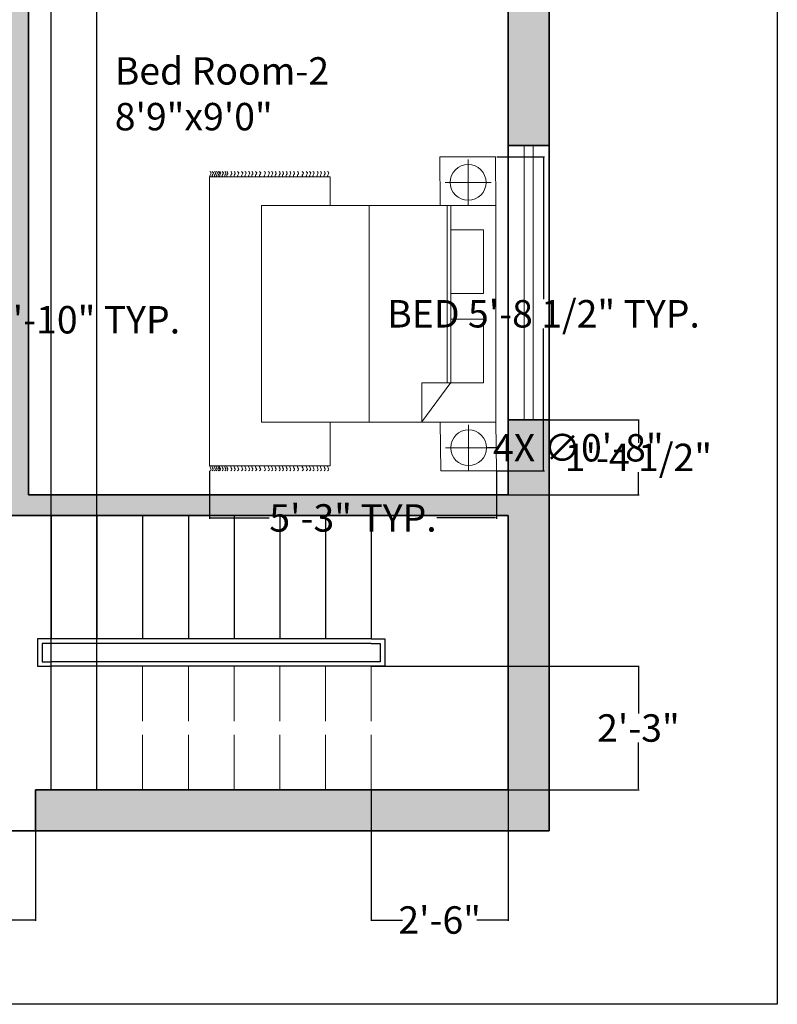
# Model space of a CAD drawing. Units: inches. Extents: x 335 to 688, y 1043 to 1486.
# Tile 2 of 7: x 515 to 681, y 1043 to 1258. Entities that reach past the tile are written whole.
import ezdxf

# ---------------------------------------------------------------- set-up
doc = ezdxf.new("R2010")
doc.units = ezdxf.units.IN
doc.header["$MEASUREMENT"] = 0
doc.linetypes.add('ACAD_ISO02W100', pattern=[15, 12, -3])
for name, color, linetype, lineweight in [('A-ANNO-DIMS', 2, 'Continuous', 18), ('A-ANNO-TTLB', 7, 'Continuous', 25), ('A-AREA-IDEN', 7, 'Continuous', 18), ('A-FLOR-STRS', 7, 'Continuous', 25), ('A-FLOR-STRS-HIDN', 7, 'ACAD_ISO02W100', 18), ('A-FURN', 8, 'Continuous', 18), ('A-GLAZ', 4, 'Continuous', 18), ('A-WALL', 7, 'Continuous', 35), ('A-WALL-PATT', 252, 'Continuous', 13)]:
    doc.layers.add(name, color=color, linetype=linetype, lineweight=lineweight)
doc.styles.get("Standard").update_dxf_attribs({"font": 'arial.ttf'})
doc.dimstyles.get("Standard").update_dxf_attribs({"dimtxt": 6, "dimasz": 0.18, "dimexe": 0.18, "dimexo": 0.0625, "dimgap": 0.09, "dimtad": 0, "dimtih": 1, "dimtoh": 1, "dimdec": 1, "dimzin": 0, "dimdsep": 46, "dimlunit": 3, "dimtxsty": 'Standard', "dimcen": 0.09, "dimadec": 0, "dimazin": 0, "dimtfac": 1, "dimtdec": 1, "dimtofl": 0, "dimtmove": 0, "dimatfit": 3, "dimfxl": 1, "dimtolj": 1, "dimtzin": 0, "dimarcsym": 0})

# ---------------------------------------------------------------- blocks, each defined once
blk = doc.blocks.new('BED-DOUBLE-WITH-NIGHTSTANDS')
for p, q in [((56.59, 58.08), (56.59, 68.14)), ((0, 64.35), (26.37, 64.35)), ((0, 1.12), (0, 64.35)), ((26.37, 64.35), (26.37, 58.06)), ((61.62, 63.11), (51.56, 63.11)), ((34.96, 10.66), (34.96, 58.08)), ((52, 19.27), (52, 58.08)), ((52.82, 19.32), (52.82, 58.08)), ((52.82, 19.32), (46.47, 10.71)), ((52.82, 19.27), (46.47, 19.27)), ((46.47, 19.27), (46.47, 10.71)), ((26.37, 10.66), (26.37, 1.12)), ((56.69, 0.03), (56.69, 10.09)), ((61.72, 5.06), (51.66, 5.06)), ((26.37, 1.12), (0, 1.12))]:
    blk.add_line(p, q)
for points in [[(50.39, 68.71), (50.5, 58.08), (62.68, 58.08), (62.58, 68.71)], [(62.68, 10.66), (11.37, 10.66), (11.37, 58.08), (62.68, 58.08)], [(59.98, 38.83), (52.82, 38.83), (52.82, 52.73), (59.98, 52.73)], [(59.98, 19.27), (52.82, 19.27), (52.82, 33.16), (59.98, 33.16)], [(50.5, 10.66), (50.6, 0.03), (62.78, 0.03), (62.68, 10.66)]]:
    blk.add_lwpolyline(points, close=True)
for centre in [(56.59, 63.11), (56.69, 5.06)]:
    blk.add_circle(centre, 3.92)
for points, knots in [([(0.07, 65.48), (0.19, 65.39), (0.43, 65.19), (0.19, 64.85), (0.02, 64.57), (0.13, 64.42), (0.18, 64.35)], [0, 0, 0, 0, 0.400747, 0.791423, 1.067667, 1.29709, 1.29709, 1.29709, 1.29709]), ([(0.57, 65.48), (0.7, 65.39), (0.94, 65.19), (0.7, 64.85), (0.52, 64.57), (0.63, 64.42), (0.68, 64.35)], [0, 0, 0, 0, 0.400747, 0.791423, 1.067667, 1.29709, 1.29709, 1.29709, 1.29709]), ([(1.06, 65.48), (1.18, 65.39), (1.42, 65.19), (1.18, 64.85), (1.01, 64.57), (1.11, 64.42), (1.16, 64.35)], [0, 0, 0, 0, 0.400747, 0.791423, 1.067667, 1.29709, 1.29709, 1.29709, 1.29709]), ([(1.46, 65.48), (1.58, 65.39), (1.82, 65.19), (1.58, 64.85), (1.41, 64.57), (1.51, 64.42), (1.56, 64.35)], [0, 0, 0, 0, 0.400747, 0.791423, 1.067667, 1.29709, 1.29709, 1.29709, 1.29709]), ([(1.88, 65.48), (2, 65.39), (2.24, 65.19), (2, 64.85), (1.82, 64.57), (1.93, 64.42), (1.98, 64.35)], [0, 0, 0, 0, 0.400747, 0.791423, 1.067667, 1.29709, 1.29709, 1.29709, 1.29709]), ([(2.18, 65.48), (2.31, 65.39), (2.55, 65.19), (2.31, 64.85), (2.13, 64.57), (2.24, 64.42), (2.29, 64.35)], [0, 0, 0, 0, 0.400747, 0.791423, 1.067667, 1.29709, 1.29709, 1.29709, 1.29709]), ([(2.76, 65.48), (2.88, 65.39), (3.12, 65.19), (2.88, 64.85), (2.71, 64.57), (2.81, 64.42), (2.86, 64.35)], [0, 0, 0, 0, 0.400747, 0.791423, 1.067667, 1.29709, 1.29709, 1.29709, 1.29709]), ([(3.33, 65.48), (3.45, 65.39), (3.7, 65.19), (3.44, 64.85), (3.27, 64.57), (3.38, 64.42), (3.43, 64.35)], [0, 0, 0, 0, 0.407265, 0.802015, 1.07826, 1.307683, 1.307683, 1.307683, 1.307683]), ([(3.75, 65.48), (3.88, 65.39), (4.12, 65.19), (3.88, 64.85), (3.7, 64.57), (3.81, 64.42), (3.86, 64.35)], [0, 0, 0, 0, 0.400747, 0.791423, 1.067667, 1.29709, 1.29709, 1.29709, 1.29709]), ([(4.64, 65.48), (4.76, 65.39), (5, 65.19), (4.76, 64.85), (4.59, 64.57), (4.69, 64.42), (4.74, 64.35)], [0, 0, 0, 0, 0.400747, 0.791423, 1.067667, 1.29709, 1.29709, 1.29709, 1.29709]), ([(5.36, 65.48), (5.49, 65.39), (5.73, 65.19), (5.49, 64.85), (5.31, 64.57), (5.42, 64.42), (5.47, 64.35)], [0, 0, 0, 0, 0.400747, 0.791423, 1.067667, 1.29709, 1.29709, 1.29709, 1.29709]), ([(6.12, 65.48), (6.24, 65.39), (6.48, 65.19), (6.24, 64.85), (6.07, 64.57), (6.17, 64.42), (6.22, 64.35)], [0, 0, 0, 0, 0.400747, 0.791423, 1.067667, 1.29709, 1.29709, 1.29709, 1.29709]), ([(7, 65.48), (7.12, 65.39), (7.36, 65.19), (7.12, 64.85), (6.95, 64.57), (7.05, 64.42), (7.1, 64.35)], [0, 0, 0, 0, 0.400747, 0.791423, 1.067667, 1.29709, 1.29709, 1.29709, 1.29709]), ([(7.73, 65.48), (7.85, 65.39), (8.09, 65.19), (7.85, 64.85), (7.68, 64.57), (7.78, 64.42), (7.83, 64.35)], [0, 0, 0, 0, 0.400747, 0.791423, 1.067667, 1.29709, 1.29709, 1.29709, 1.29709]), ([(8.54, 65.48), (8.66, 65.39), (8.9, 65.19), (8.66, 64.85), (8.49, 64.57), (8.6, 64.42), (8.65, 64.35)], [0, 0, 0, 0, 0.400747, 0.791423, 1.067667, 1.29709, 1.29709, 1.29709, 1.29709]), ([(9.23, 65.48), (9.35, 65.39), (9.59, 65.19), (9.35, 64.85), (9.18, 64.57), (9.29, 64.42), (9.34, 64.35)], [0, 0, 0, 0, 0.400747, 0.791423, 1.067667, 1.29709, 1.29709, 1.29709, 1.29709]), ([(10.05, 65.48), (10.17, 65.39), (10.41, 65.19), (10.17, 64.85), (10, 64.57), (10.1, 64.42), (10.15, 64.35)], [0, 0, 0, 0, 0.400747, 0.791423, 1.067667, 1.29709, 1.29709, 1.29709, 1.29709]), ([(10.93, 65.48), (11.05, 65.39), (11.29, 65.19), (11.05, 64.85), (10.88, 64.57), (10.99, 64.42), (11.03, 64.35)], [0, 0, 0, 0, 0.400747, 0.791423, 1.067667, 1.29709, 1.29709, 1.29709, 1.29709]), ([(11.97, 65.48), (12.09, 65.39), (12.33, 65.19), (12.09, 64.85), (11.92, 64.57), (12.02, 64.42), (12.07, 64.35)], [0, 0, 0, 0, 0.400747, 0.791423, 1.067667, 1.29709, 1.29709, 1.29709, 1.29709]), ([(12.85, 65.48), (12.97, 65.39), (13.21, 65.19), (12.97, 64.85), (12.8, 64.57), (12.9, 64.42), (12.95, 64.35)], [0, 0, 0, 0, 0.400747, 0.791423, 1.067667, 1.29709, 1.29709, 1.29709, 1.29709]), ([(13.58, 65.48), (13.7, 65.39), (13.94, 65.19), (13.7, 64.85), (13.53, 64.57), (13.63, 64.42), (13.68, 64.35)], [0, 0, 0, 0, 0.400747, 0.791423, 1.067667, 1.29709, 1.29709, 1.29709, 1.29709]), ([(14.33, 65.48), (14.45, 65.39), (14.69, 65.19), (14.45, 64.85), (14.28, 64.57), (14.38, 64.42), (14.43, 64.35)], [0, 0, 0, 0, 0.400747, 0.791423, 1.067667, 1.29709, 1.29709, 1.29709, 1.29709]), ([(15.21, 65.48), (15.33, 65.39), (15.57, 65.19), (15.33, 64.85), (15.16, 64.57), (15.27, 64.42), (15.32, 64.35)], [0, 0, 0, 0, 0.400747, 0.791423, 1.067667, 1.29709, 1.29709, 1.29709, 1.29709]), ([(15.94, 65.48), (16.06, 65.39), (16.3, 65.19), (16.06, 64.85), (15.89, 64.57), (16, 64.42), (16.04, 64.35)], [0, 0, 0, 0, 0.400747, 0.791423, 1.067667, 1.29709, 1.29709, 1.29709, 1.29709]), ([(16.76, 65.48), (16.88, 65.39), (17.12, 65.19), (16.88, 64.85), (16.7, 64.57), (16.81, 64.42), (16.86, 64.35)], [0, 0, 0, 0, 0.400747, 0.791423, 1.067667, 1.29709, 1.29709, 1.29709, 1.29709]), ([(17.53, 65.48), (17.65, 65.39), (17.89, 65.19), (17.65, 64.85), (17.48, 64.57), (17.59, 64.42), (17.64, 64.35)], [0, 0, 0, 0, 0.400747, 0.791423, 1.067667, 1.29709, 1.29709, 1.29709, 1.29709]), ([(18.35, 65.48), (18.47, 65.39), (18.71, 65.19), (18.47, 64.85), (18.3, 64.57), (18.4, 64.42), (18.45, 64.35)], [0, 0, 0, 0, 0.400747, 0.791423, 1.067667, 1.29709, 1.29709, 1.29709, 1.29709]), ([(19.23, 65.48), (19.35, 65.39), (19.59, 65.19), (19.35, 64.85), (19.18, 64.57), (19.29, 64.42), (19.33, 64.35)], [0, 0, 0, 0, 0.400747, 0.791423, 1.067667, 1.29709, 1.29709, 1.29709, 1.29709]), ([(20.27, 65.48), (20.39, 65.39), (20.63, 65.19), (20.39, 64.85), (20.22, 64.57), (20.32, 64.42), (20.37, 64.35)], [0, 0, 0, 0, 0.400747, 0.791423, 1.067667, 1.29709, 1.29709, 1.29709, 1.29709]), ([(21.15, 65.48), (21.27, 65.39), (21.51, 65.19), (21.27, 64.85), (21.1, 64.57), (21.21, 64.42), (21.25, 64.35)], [0, 0, 0, 0, 0.400747, 0.791423, 1.067667, 1.29709, 1.29709, 1.29709, 1.29709]), ([(21.88, 65.48), (22, 65.39), (22.24, 65.19), (22, 64.85), (21.83, 64.57), (21.93, 64.42), (21.98, 64.35)], [0, 0, 0, 0, 0.400747, 0.791423, 1.067667, 1.29709, 1.29709, 1.29709, 1.29709]), ([(22.63, 65.48), (22.75, 65.39), (22.99, 65.19), (22.75, 64.85), (22.58, 64.57), (22.69, 64.42), (22.73, 64.35)], [0, 0, 0, 0, 0.400747, 0.791423, 1.067667, 1.29709, 1.29709, 1.29709, 1.29709]), ([(23.51, 65.48), (23.63, 65.39), (23.87, 65.19), (23.63, 64.85), (23.46, 64.57), (23.57, 64.42), (23.62, 64.35)], [0, 0, 0, 0, 0.400747, 0.791423, 1.067667, 1.29709, 1.29709, 1.29709, 1.29709]), ([(24.24, 65.48), (24.36, 65.39), (24.6, 65.19), (24.36, 64.85), (24.19, 64.57), (24.3, 64.42), (24.34, 64.35)], [0, 0, 0, 0, 0.400747, 0.791423, 1.067667, 1.29709, 1.29709, 1.29709, 1.29709]), ([(25.06, 65.48), (25.18, 65.39), (25.42, 65.19), (25.18, 64.85), (25.01, 64.57), (25.11, 64.42), (25.16, 64.35)], [0, 0, 0, 0, 0.400747, 0.791423, 1.067667, 1.29709, 1.29709, 1.29709, 1.29709]), ([(25.84, 65.48), (25.96, 65.39), (26.2, 65.19), (25.96, 64.85), (25.78, 64.57), (25.89, 64.42), (25.94, 64.35)], [0, 0, 0, 0, 0.400747, 0.791423, 1.067667, 1.29709, 1.29709, 1.29709, 1.29709]), ([(0.07, 0), (0.19, 0.1), (0.43, 0.29), (0.19, 0.63), (0.02, 0.91), (0.13, 1.06), (0.18, 1.13)], [0, 0, 0, 0, 0.400747, 0.791423, 1.067667, 1.29709, 1.29709, 1.29709, 1.29709]), ([(0.55, 0), (0.67, 0.1), (0.91, 0.29), (0.67, 0.63), (0.49, 0.91), (0.6, 1.06), (0.65, 1.13)], [0, 0, 0, 0, 0.400747, 0.791423, 1.067667, 1.29709, 1.29709, 1.29709, 1.29709]), ([(1.03, 0), (1.15, 0.1), (1.39, 0.29), (1.15, 0.63), (0.98, 0.91), (1.09, 1.06), (1.13, 1.13)], [0, 0, 0, 0, 0.400747, 0.791423, 1.067667, 1.29709, 1.29709, 1.29709, 1.29709]), ([(1.43, 0), (1.55, 0.1), (1.79, 0.29), (1.55, 0.63), (1.38, 0.91), (1.48, 1.06), (1.53, 1.13)], [0, 0, 0, 0, 0.400747, 0.791423, 1.067667, 1.29709, 1.29709, 1.29709, 1.29709]), ([(1.85, 0), (1.97, 0.1), (2.21, 0.29), (1.97, 0.63), (1.8, 0.91), (1.9, 1.05), (1.94, 1.12)], [0, 0, 0, 0, 0.400747, 0.791423, 1.067667, 1.283686, 1.283686, 1.283686, 1.283686]), ([(2.16, 0), (2.28, 0.1), (2.52, 0.29), (2.28, 0.63), (2.11, 0.91), (2.21, 1.05), (2.25, 1.12)], [0, 0, 0, 0, 0.400747, 0.791423, 1.067667, 1.283686, 1.283686, 1.283686, 1.283686]), ([(2.73, 0), (2.85, 0.1), (3.09, 0.29), (2.85, 0.63), (2.68, 0.91), (2.78, 1.05), (2.82, 1.12)], [0, 0, 0, 0, 0.400747, 0.791423, 1.067667, 1.283686, 1.283686, 1.283686, 1.283686]), ([(3.33, 0), (3.45, 0.1), (3.69, 0.29), (3.45, 0.63), (3.28, 0.91), (3.38, 1.05), (3.42, 1.12)], [0, 0, 0, 0, 0.402903, 0.794912, 1.071156, 1.287177, 1.287177, 1.287177, 1.287177]), ([(3.75, 0), (3.88, 0.1), (4.12, 0.29), (3.88, 0.63), (3.7, 0.91), (3.81, 1.05), (3.85, 1.12)], [0, 0, 0, 0, 0.400747, 0.791423, 1.067667, 1.283686, 1.283686, 1.283686, 1.283686]), ([(4.64, 0), (4.76, 0.1), (5, 0.29), (4.76, 0.63), (4.59, 0.91), (4.69, 1.05), (4.73, 1.12)], [0, 0, 0, 0, 0.400747, 0.791423, 1.067667, 1.283686, 1.283686, 1.283686, 1.283686]), ([(5.36, 0), (5.49, 0.1), (5.73, 0.29), (5.49, 0.63), (5.31, 0.91), (5.42, 1.06), (5.47, 1.13)], [0, 0, 0, 0, 0.400747, 0.791423, 1.067667, 1.29709, 1.29709, 1.29709, 1.29709]), ([(6.12, 0), (6.24, 0.1), (6.48, 0.29), (6.24, 0.63), (6.07, 0.91), (6.17, 1.06), (6.22, 1.13)], [0, 0, 0, 0, 0.400747, 0.791423, 1.067667, 1.29709, 1.29709, 1.29709, 1.29709]), ([(7, 0), (7.12, 0.1), (7.36, 0.29), (7.12, 0.63), (6.95, 0.91), (7.05, 1.06), (7.1, 1.13)], [0, 0, 0, 0, 0.400747, 0.791423, 1.067667, 1.29709, 1.29709, 1.29709, 1.29709]), ([(7.73, 0), (7.85, 0.1), (8.09, 0.29), (7.85, 0.63), (7.68, 0.91), (7.78, 1.06), (7.83, 1.13)], [0, 0, 0, 0, 0.400747, 0.791423, 1.067667, 1.29709, 1.29709, 1.29709, 1.29709]), ([(8.54, 0), (8.66, 0.1), (8.9, 0.29), (8.66, 0.63), (8.49, 0.91), (8.6, 1.06), (8.65, 1.13)], [0, 0, 0, 0, 0.400747, 0.791423, 1.067667, 1.29709, 1.29709, 1.29709, 1.29709]), ([(9.23, 0), (9.35, 0.1), (9.59, 0.29), (9.35, 0.63), (9.18, 0.91), (9.29, 1.06), (9.34, 1.13)], [0, 0, 0, 0, 0.400747, 0.791423, 1.067667, 1.29709, 1.29709, 1.29709, 1.29709]), ([(10.05, 0), (10.17, 0.1), (10.41, 0.29), (10.17, 0.63), (10, 0.91), (10.1, 1.06), (10.15, 1.13)], [0, 0, 0, 0, 0.400747, 0.791423, 1.067667, 1.29709, 1.29709, 1.29709, 1.29709]), ([(10.93, 0), (11.05, 0.1), (11.29, 0.29), (11.05, 0.63), (10.88, 0.91), (10.99, 1.06), (11.03, 1.13)], [0, 0, 0, 0, 0.400747, 0.791423, 1.067667, 1.29709, 1.29709, 1.29709, 1.29709]), ([(11.97, 0), (12.09, 0.1), (12.33, 0.29), (12.09, 0.63), (11.92, 0.91), (12.02, 1.06), (12.07, 1.13)], [0, 0, 0, 0, 0.400747, 0.791423, 1.067667, 1.29709, 1.29709, 1.29709, 1.29709]), ([(12.85, 0), (12.97, 0.1), (13.21, 0.29), (12.97, 0.63), (12.8, 0.91), (12.9, 1.06), (12.95, 1.13)], [0, 0, 0, 0, 0.400747, 0.791423, 1.067667, 1.29709, 1.29709, 1.29709, 1.29709]), ([(13.58, 0), (13.7, 0.1), (13.94, 0.29), (13.7, 0.63), (13.53, 0.91), (13.63, 1.06), (13.68, 1.13)], [0, 0, 0, 0, 0.400747, 0.791423, 1.067667, 1.29709, 1.29709, 1.29709, 1.29709]), ([(14.33, 0), (14.45, 0.1), (14.69, 0.29), (14.45, 0.63), (14.28, 0.91), (14.38, 1.06), (14.43, 1.13)], [0, 0, 0, 0, 0.400747, 0.791423, 1.067667, 1.29709, 1.29709, 1.29709, 1.29709]), ([(15.21, 0), (15.33, 0.1), (15.57, 0.29), (15.33, 0.63), (15.16, 0.91), (15.27, 1.06), (15.32, 1.13)], [0, 0, 0, 0, 0.400747, 0.791423, 1.067667, 1.29709, 1.29709, 1.29709, 1.29709]), ([(15.94, 0), (16.06, 0.1), (16.3, 0.29), (16.06, 0.63), (15.89, 0.91), (16, 1.06), (16.04, 1.13)], [0, 0, 0, 0, 0.400747, 0.791423, 1.067667, 1.29709, 1.29709, 1.29709, 1.29709]), ([(16.76, 0), (16.88, 0.1), (17.12, 0.29), (16.88, 0.63), (16.7, 0.91), (16.81, 1.06), (16.86, 1.13)], [0, 0, 0, 0, 0.400747, 0.791423, 1.067667, 1.29709, 1.29709, 1.29709, 1.29709]), ([(17.53, 0), (17.65, 0.1), (17.89, 0.29), (17.65, 0.63), (17.48, 0.91), (17.59, 1.06), (17.64, 1.13)], [0, 0, 0, 0, 0.400747, 0.791423, 1.067667, 1.29709, 1.29709, 1.29709, 1.29709]), ([(18.35, 0), (18.47, 0.1), (18.71, 0.29), (18.47, 0.63), (18.3, 0.91), (18.4, 1.06), (18.45, 1.13)], [0, 0, 0, 0, 0.400747, 0.791423, 1.067667, 1.29709, 1.29709, 1.29709, 1.29709]), ([(19.23, 0), (19.35, 0.1), (19.59, 0.29), (19.35, 0.63), (19.18, 0.91), (19.29, 1.06), (19.33, 1.13)], [0, 0, 0, 0, 0.400747, 0.791423, 1.067667, 1.29709, 1.29709, 1.29709, 1.29709]), ([(20.27, 0), (20.39, 0.1), (20.63, 0.29), (20.39, 0.63), (20.22, 0.91), (20.32, 1.06), (20.37, 1.13)], [0, 0, 0, 0, 0.400747, 0.791423, 1.067667, 1.29709, 1.29709, 1.29709, 1.29709]), ([(21.15, 0), (21.27, 0.1), (21.51, 0.29), (21.27, 0.63), (21.1, 0.91), (21.21, 1.06), (21.25, 1.13)], [0, 0, 0, 0, 0.400747, 0.791423, 1.067667, 1.29709, 1.29709, 1.29709, 1.29709]), ([(21.88, 0), (22, 0.1), (22.24, 0.29), (22, 0.63), (21.83, 0.91), (21.93, 1.06), (21.98, 1.13)], [0, 0, 0, 0, 0.400747, 0.791423, 1.067667, 1.29709, 1.29709, 1.29709, 1.29709]), ([(22.63, 0), (22.75, 0.1), (22.99, 0.29), (22.75, 0.63), (22.58, 0.91), (22.69, 1.06), (22.73, 1.13)], [0, 0, 0, 0, 0.400747, 0.791423, 1.067667, 1.29709, 1.29709, 1.29709, 1.29709]), ([(23.51, 0), (23.63, 0.1), (23.87, 0.29), (23.63, 0.63), (23.46, 0.91), (23.57, 1.06), (23.62, 1.13)], [0, 0, 0, 0, 0.400747, 0.791423, 1.067667, 1.29709, 1.29709, 1.29709, 1.29709]), ([(24.24, 0), (24.36, 0.1), (24.6, 0.29), (24.36, 0.63), (24.19, 0.91), (24.3, 1.06), (24.34, 1.13)], [0, 0, 0, 0, 0.400747, 0.791423, 1.067667, 1.29709, 1.29709, 1.29709, 1.29709]), ([(25.06, 0), (25.18, 0.1), (25.42, 0.29), (25.18, 0.63), (25.01, 0.91), (25.11, 1.06), (25.16, 1.13)], [0, 0, 0, 0, 0.400747, 0.791423, 1.067667, 1.29709, 1.29709, 1.29709, 1.29709]), ([(25.84, 0), (25.96, 0.1), (26.2, 0.29), (25.96, 0.63), (25.78, 0.91), (25.89, 1.06), (25.94, 1.13)], [0, 0, 0, 0, 0.400747, 0.791423, 1.067667, 1.29709, 1.29709, 1.29709, 1.29709])]:
    blk.add_open_spline(points, degree=3, knots=knots)
blk = doc.blocks.new('WIN-60IN')
for p, q in [((0, 0), (0, 60)), ((3.5, 0), (3.5, 60)), ((5.5, 60), (5.5, 0)), ((9, 60), (9, 0))]:
    blk.add_line(p, q)
blk = doc.blocks.new('*D15')
at = {"layer": 'A-ANNO-DIMS', "color": 0, "lineweight": -2, "transparency": 16777216}
for p, q in [((619.61, 1228.43), (630.03, 1228.43)), ((629.85, 1228.25), (629.85, 1197.27)), ((629.85, 1159.9), (629.85, 1190.88)), ((619.61, 1159.72), (630.03, 1159.72))]:
    blk.add_line(p, q, dxfattribs=at)
at = {"layer": 'A-ANNO-DIMS', "color": 0, "transparency": 16777216}
for points in [[(629.82, 1228.25), (629.88, 1228.25), (629.85, 1228.43)], [(629.82, 1159.9), (629.88, 1159.9), (629.85, 1159.72)]]:
    blk.add_solid(points, dxfattribs=at)
at = {"layer": 'Defpoints', "color": 0, "transparency": 16777216}
for p in [(619.54, 1228.43), (629.85, 1228.43), (619.54, 1159.72)]:
    blk.add_point(p, dxfattribs=at)
at = {"layer": 'A-ANNO-DIMS', "color": 0, "transparency": 16777216, "insert": (629.85, 1194.08), "char_height": 6, "attachment_point": 5}
blk.add_mtext('\\A1;BED 5\'-8 1/2" TYP.', dxfattribs=at)
blk = doc.blocks.new('*D16')
at = {"layer": 'A-ANNO-DIMS', "color": 0, "lineweight": -2, "transparency": 16777216}
for p, q in [((556.76, 1159.66), (556.76, 1149.24)), ((619.54, 1159.66), (619.54, 1149.24)), ((556.94, 1149.42), (569.78, 1149.42)), ((619.36, 1149.42), (606.53, 1149.42))]:
    blk.add_line(p, q, dxfattribs=at)
at = {"layer": 'A-ANNO-DIMS', "color": 0, "transparency": 16777216}
for points in [[(556.94, 1149.45), (556.94, 1149.39), (556.76, 1149.42)], [(619.36, 1149.45), (619.36, 1149.39), (619.54, 1149.42)]]:
    blk.add_solid(points, dxfattribs=at)
at = {"layer": 'Defpoints', "color": 0, "transparency": 16777216}
for p in [(556.76, 1159.72), (619.54, 1159.72), (619.54, 1149.42)]:
    blk.add_point(p, dxfattribs=at)
at = {"layer": 'A-ANNO-DIMS', "color": 0, "transparency": 16777216, "insert": (588.15, 1149.42), "char_height": 6, "attachment_point": 5}
blk.add_mtext('\\A1;5\'-3" TYP.', dxfattribs=at)
blk = doc.blocks.new('*D20')
at = {"layer": 'A-ANNO-DIMS', "color": 0, "lineweight": -2, "transparency": 16777216}
for p, q in [((486.89, 1200.97), (486.89, 1192.6)), ((509.12, 1200.97), (509.12, 1192.6)), ((487.07, 1192.78), (508.94, 1192.78)), ((509.12, 1192.78), (509.3, 1192.78))]:
    blk.add_line(p, q, dxfattribs=at)
at = {"layer": 'A-ANNO-DIMS', "color": 0, "transparency": 16777216}
for points in [[(487.07, 1192.81), (487.07, 1192.75), (486.89, 1192.78)], [(508.94, 1192.81), (508.94, 1192.75), (509.12, 1192.78)]]:
    blk.add_solid(points, dxfattribs=at)
at = {"layer": 'Defpoints', "color": 0, "transparency": 16777216}
for p in [(486.89, 1201.04), (509.12, 1201.04), (509.12, 1192.78)]:
    blk.add_point(p, dxfattribs=at)
at = {"layer": 'A-ANNO-DIMS', "color": 0, "transparency": 16777216, "insert": (529.72, 1192.78), "char_height": 6, "attachment_point": 5}
blk.add_mtext('\\A1;1\'-10" TYP.', dxfattribs=at)
blk = doc.blocks.new('*D51')
at = {"layer": 'A-ANNO-DIMS', "color": 0, "lineweight": -2, "transparency": 16777216}
for p, q in [((622.17, 1170.86), (650.79, 1170.86)), ((650.61, 1170.68), (650.61, 1165.86)), ((650.61, 1154.65), (650.61, 1159.47)), ((622.17, 1154.47), (650.79, 1154.47))]:
    blk.add_line(p, q, dxfattribs=at)
at = {"layer": 'A-ANNO-DIMS', "color": 0, "transparency": 16777216}
for points in [[(650.58, 1170.68), (650.64, 1170.68), (650.61, 1170.86)], [(650.58, 1154.65), (650.64, 1154.65), (650.61, 1154.47)]]:
    blk.add_solid(points, dxfattribs=at)
at = {"layer": 'Defpoints', "color": 0, "transparency": 16777216}
for p in [(622.11, 1170.86), (650.61, 1170.86), (622.11, 1154.47)]:
    blk.add_point(p, dxfattribs=at)
at = {"layer": 'A-ANNO-DIMS', "color": 0, "transparency": 16777216, "insert": (650.61, 1162.66), "char_height": 6, "attachment_point": 5}
blk.add_mtext('\\A1;1\'-4 1/2"', dxfattribs=at)
blk = doc.blocks.new('*D56')
at = {"layer": 'A-ANNO-DIMS', "color": 0, "lineweight": -2, "transparency": 16777216}
for p, q in [((467.19, 1080.9), (467.19, 1061.29)), ((518.67, 1080.9), (518.67, 1061.29)), ((467.37, 1061.47), (477.75, 1061.47)), ((518.49, 1061.47), (508.1, 1061.47))]:
    blk.add_line(p, q, dxfattribs=at)
at = {"layer": 'A-ANNO-DIMS', "color": 0, "transparency": 16777216}
for points in [[(467.37, 1061.5), (467.37, 1061.44), (467.19, 1061.47)], [(518.49, 1061.5), (518.49, 1061.44), (518.67, 1061.47)]]:
    blk.add_solid(points, dxfattribs=at)
at = {"layer": 'Defpoints', "color": 0, "transparency": 16777216}
for p in [(467.19, 1080.97), (518.67, 1080.97), (518.67, 1061.47)]:
    blk.add_point(p, dxfattribs=at)
at = {"layer": 'A-ANNO-DIMS', "color": 0, "transparency": 16777216, "insert": (492.93, 1061.47), "char_height": 6, "attachment_point": 5}
blk.add_mtext('\\A1;4\'-3 1/2"', dxfattribs=at)
blk = doc.blocks.new('*D57')
at = {"layer": 'A-ANNO-DIMS', "color": 0, "lineweight": -2, "transparency": 16777216}
for p, q in [((522.11, 1090.03), (522.11, 1460.65)), ((522.29, 1460.47), (531.93, 1460.47)), ((532.11, 1090.03), (532.11, 1460.65)), ((532.11, 1460.47), (532.29, 1460.47))]:
    blk.add_line(p, q, dxfattribs=at)
at = {"layer": 'A-ANNO-DIMS', "color": 0, "transparency": 16777216}
for points in [[(522.29, 1460.5), (522.29, 1460.44), (522.11, 1460.47)], [(531.93, 1460.5), (531.93, 1460.44), (532.11, 1460.47)]]:
    blk.add_solid(points, dxfattribs=at)
at = {"layer": 'Defpoints', "color": 0, "transparency": 16777216}
for p in [(532.11, 1460.47), (522.11, 1089.97), (532.11, 1089.97)]:
    blk.add_point(p, dxfattribs=at)
at = {"layer": 'A-ANNO-DIMS', "color": 0, "transparency": 16777216, "insert": (542.68, 1460.47), "char_height": 6, "attachment_point": 5}
blk.add_mtext('\\A1;0\'-10"', dxfattribs=at)
blk = doc.blocks.new('*D58')
at = {"layer": 'A-ANNO-DIMS', "color": 0, "lineweight": -2, "transparency": 16777216}
for p, q in [((592.11, 1089.9), (592.11, 1061.29)), ((622.11, 1089.9), (622.11, 1061.29)), ((592.29, 1061.47), (598.99, 1061.47)), ((621.93, 1061.47), (615.22, 1061.47))]:
    blk.add_line(p, q, dxfattribs=at)
at = {"layer": 'A-ANNO-DIMS', "color": 0, "transparency": 16777216}
for points in [[(592.29, 1061.5), (592.29, 1061.44), (592.11, 1061.47)], [(621.93, 1061.5), (621.93, 1061.44), (622.11, 1061.47)]]:
    blk.add_solid(points, dxfattribs=at)
at = {"layer": 'Defpoints', "color": 0, "transparency": 16777216}
for p in [(592.11, 1089.97), (622.11, 1089.97), (622.11, 1061.47)]:
    blk.add_point(p, dxfattribs=at)
at = {"layer": 'A-ANNO-DIMS', "color": 0, "transparency": 16777216, "insert": (607.11, 1061.47), "char_height": 6, "attachment_point": 5}
blk.add_mtext('\\A1;2\'-6"', dxfattribs=at)
blk = doc.blocks.new('*D59')
at = {"layer": 'A-ANNO-DIMS', "color": 0, "lineweight": -2, "transparency": 16777216}
for p, q in [((592.17, 1116.97), (650.79, 1116.97)), ((650.61, 1116.79), (650.61, 1106.62)), ((650.61, 1090.15), (650.61, 1100.31)), ((592.17, 1089.97), (650.79, 1089.97))]:
    blk.add_line(p, q, dxfattribs=at)
at = {"layer": 'A-ANNO-DIMS', "color": 0, "transparency": 16777216}
for points in [[(650.58, 1116.79), (650.64, 1116.79), (650.61, 1116.97)], [(650.58, 1090.15), (650.64, 1090.15), (650.61, 1089.97)]]:
    blk.add_solid(points, dxfattribs=at)
at = {"layer": 'Defpoints', "color": 0, "transparency": 16777216}
for p in [(592.11, 1116.97), (650.61, 1116.97), (592.11, 1089.97)]:
    blk.add_point(p, dxfattribs=at)
at = {"layer": 'A-ANNO-DIMS', "color": 0, "transparency": 16777216, "insert": (650.61, 1103.47), "char_height": 6, "attachment_point": 5}
blk.add_mtext('\\A1;2\'-3"', dxfattribs=at)
blk = doc.blocks.new('*D68')
at = {"layer": 'A-ANNO-DIMS', "color": 0, "lineweight": -2, "transparency": 16777216}
for p, q in [((613.36, 1164.78), (613.54, 1164.78)), ((613.45, 1164.69), (613.45, 1164.87)), ((619.73, 1164.78), (617.55, 1164.78))]:
    blk.add_line(p, q, dxfattribs=at)
at = {"layer": 'A-ANNO-DIMS', "color": 0, "transparency": 16777216}
blk.add_solid([(617.55, 1164.81), (617.55, 1164.75), (617.37, 1164.78)], dxfattribs=at)
at = {"layer": 'Defpoints', "color": 0, "transparency": 16777216}
for p in [(609.53, 1164.78), (617.37, 1164.78)]:
    blk.add_point(p, dxfattribs=at)
at = {"layer": 'A-ANNO-DIMS', "color": 0, "transparency": 16777216, "insert": (637.46, 1164.78), "char_height": 6, "attachment_point": 5}
blk.add_mtext('\\A1;4X ∅0\'-8"', dxfattribs=at)

msp = doc.modelspace()

# ---------------------------------------------------------------- hatches: boundary and pattern name
at = {"layer": 'A-WALL-PATT'}
h = msp.add_hatch(color=256, dxfattribs=at)
h.dxf.hatch_style = 1
h.paths.add_polyline_path([(478.71, 1440.97), (391.11, 1440.97), (391.11, 1411.42), (400.11, 1411.42), (400.11, 1431.97), (466.11, 1431.97), (466.11, 1347.97), (466.11, 1343.47), (470.61, 1343.47), (470.61, 1367.47), (512.61, 1367.47), (512.61, 1350.97), (517.11, 1350.97), (517.11, 1372.97), (512.61, 1372.97), (512.61, 1371.97), (470.61, 1371.97), (470.61, 1431.97), (478.71, 1431.97)])
h.paths.add_polyline_path([(631.11, 1440.97), (502.71, 1440.97), (502.71, 1431.97), (512.61, 1431.97), (512.61, 1404.97), (517.11, 1404.97), (517.11, 1431.97), (622.11, 1431.97), (622.11, 1401.6), (631.11, 1401.6)])
h.paths.add_polyline_path([(631.11, 1341.6), (622.11, 1341.6), (622.11, 1313.47), (517.11, 1313.47), (517.11, 1314.47), (512.61, 1314.47), (512.61, 1313.47), (512.61, 1307.97), (517.11, 1307.97), (517.11, 1308.97), (553.11, 1308.97), (553.11, 1262.47), (558.61, 1262.47), (558.61, 1266.97), (557.61, 1266.97), (557.61, 1308.97), (622.11, 1308.97), (622.11, 1297.63), (631.11, 1297.63)])
h.paths.add_polyline_path([(631.11, 1273.63), (622.11, 1273.63), (622.11, 1266.97), (590.61, 1266.97), (590.61, 1262.47), (622.11, 1262.47), (622.11, 1230.86), (631.11, 1230.86)])
h.paths.add_polyline_path([(400.11, 1253.85), (391.11, 1253.85), (391.11, 1132.26), (400.11, 1132.26), (400.11, 1149.97), (411.11, 1149.97), (411.11, 1154.47), (400.11, 1154.47)], flags=17)
h.paths.add_polyline_path([(400.11, 1375.42), (391.11, 1375.42), (391.11, 1313.85), (400.11, 1313.85), (400.11, 1343.47), (428.36, 1343.47), (428.36, 1347.97), (400.11, 1347.97)])
h = msp.add_hatch(color=256, dxfattribs=at)
h.dxf.hatch_style = 1
h.paths.add_polyline_path([(467.19, 1089.97), (464.61, 1089.97), (464.61, 1149.97), (475.61, 1149.97), (475.61, 1154.47), (459.11, 1154.47), (459.11, 1149.97), (460.11, 1149.97), (460.11, 1089.97), (400.11, 1089.97), (400.11, 1108.26), (391.11, 1108.26), (391.11, 1080.97), (467.19, 1080.97)])
h.paths.add_polyline_path([(631.11, 1170.86), (622.11, 1170.86), (622.11, 1154.47), (517.11, 1154.47), (517.11, 1271.97), (512.61, 1271.97), (512.61, 1154.47), (511.61, 1154.47), (511.61, 1149.97), (512.61, 1149.97), (622.11, 1149.97), (622.11, 1089.97), (518.67, 1089.97), (518.67, 1080.97), (631.11, 1080.97)])

# ---------------------------------------------------------------- linework, layer by layer
at = {"layer": 'A-ANNO-TTLB'}
msp.add_lwpolyline([(334.72, 1486.4), (681.01, 1486.4), (681.01, 1043.03), (334.72, 1043.03)], close=True, dxfattribs=at)
at = {"layer": 'A-FLOR-STRS'}
for p, q in [((522.11, 1149.97), (522.11, 1122.97)), ((532.11, 1149.97), (532.11, 1122.97)), ((542.11, 1149.97), (542.11, 1122.97)), ((552.11, 1149.97), (552.11, 1122.97)), ((562.11, 1149.97), (562.11, 1122.97)), ((572.11, 1149.97), (572.11, 1122.97)), ((582.11, 1149.97), (582.11, 1122.97)), ((592.11, 1149.97), (592.11, 1122.97)), ((622.11, 1149.97), (622.11, 1149.97)), ((522.11, 1122.97), (519.11, 1122.97)), ((519.11, 1122.97), (519.11, 1116.97)), ((592.11, 1122.97), (522.11, 1122.97)), ((592.11, 1122.97), (595.11, 1122.97)), ((595.11, 1122.97), (595.11, 1116.97)), ((522.11, 1121.97), (520.11, 1121.97)), ((520.11, 1121.97), (520.11, 1117.97)), ((592.11, 1121.97), (522.11, 1121.97)), ((592.11, 1121.97), (594.11, 1121.97)), ((594.11, 1121.97), (594.11, 1117.97)), ((520.11, 1117.97), (522.11, 1117.97)), ((592.11, 1117.97), (522.11, 1117.97)), ((594.11, 1117.97), (592.11, 1117.97)), ((519.11, 1116.97), (522.11, 1116.97)), ((592.11, 1116.97), (522.11, 1116.97)), ((595.11, 1116.97), (592.11, 1116.97))]:
    msp.add_line(p, q, dxfattribs=at)
at = {"layer": 'A-FLOR-STRS-HIDN'}
for p, q in [((522.11, 1116.97), (522.11, 1089.97)), ((532.11, 1116.97), (532.11, 1089.97)), ((542.11, 1116.97), (542.11, 1089.97)), ((552.11, 1116.97), (552.11, 1089.97)), ((562.11, 1116.97), (562.11, 1089.97)), ((572.11, 1116.97), (572.11, 1089.97)), ((582.11, 1116.97), (582.11, 1089.97)), ((592.11, 1116.97), (592.11, 1089.97))]:
    msp.add_line(p, q, dxfattribs=at)
at = {"layer": 'A-WALL'}
for p, q in [((631.11, 1440.97), (631.11, 1080.97)), ((517.11, 1271.97), (517.11, 1154.47)), ((622.11, 1262.47), (622.11, 1154.47)), ((622.11, 1230.86), (631.11, 1230.86)), ((631.11, 1170.86), (622.11, 1170.86)), ((517.11, 1154.47), (622.11, 1154.47)), ((464.61, 1149.97), (622.11, 1149.97)), ((622.11, 1149.97), (622.11, 1089.97)), ((518.67, 1089.97), (518.67, 1080.97)), ((518.67, 1089.97), (622.11, 1089.97)), ((391.11, 1080.97), (631.11, 1080.97)), ((518.67, 1080.97), (467.19, 1080.97))]:
    msp.add_line(p, q, dxfattribs=at)

# ---------------------------------------------------------------- block references
at = {"layer": 'A-FURN'}
msp.add_blockref('BED-DOUBLE-WITH-NIGHTSTANDS', (556.76, 1159.72), dxfattribs=at)
at = {"layer": 'A-GLAZ'}
msp.add_blockref('WIN-60IN', (622.11, 1170.86), dxfattribs=at)

# ---------------------------------------------------------------- texts
at = {"layer": 'A-AREA-IDEN', "insert": (536.01, 1250.21), "char_height": 6, "attachment_point": 1}
msp.add_mtext_dynamic_manual_height_columns('Bed Room-2\\P8\'9"x9\'0"', width=63.6169, gutter_width=1, heights=[0], dxfattribs=at)

# ---------------------------------------------------------------- dimensions: what is measured, and where the dimension line sits
at = {"layer": 'A-ANNO-DIMS'}
for base, p1, p2, picture, middle in [((532.11, 1460.47), (522.11, 1089.97), (532.11, 1089.97), '*D57', (542.68, 1460.47)), ((622.11, 1061.47), (592.11, 1089.97), (622.11, 1089.97), '*D58', (607.11, 1061.47)), ((518.67, 1061.47), (467.19, 1080.97), (518.67, 1080.97), '*D56', (492.93, 1061.47))]:
    dim = msp.add_linear_dim(base=base, p1=p1, p2=p2, dimstyle='Standard', override={"dimdec": 1, "dimlfac": 1, "dimrnd": 0, "dimzin": 1, "dimdsep": 46, "dimlunit": 4, "dimfrac": 2}, dxfattribs=at)
    dim.commit()
    dim.dimension.update_dxf_attribs({"geometry": picture, "text_midpoint": middle})
dim = msp.add_linear_dim(base=(629.85, 1228.43), p1=(619.54, 1159.72), p2=(619.54, 1228.43), angle=90, text='BED <> TYP.', dimstyle='Standard', override={"dimdec": 1, "dimlfac": 1, "dimrnd": 0, "dimzin": 1, "dimdsep": 46, "dimlunit": 4, "dimfrac": 2}, dxfattribs=at)
dim.commit()
dim.dimension.update_dxf_attribs({"geometry": '*D15', "text_midpoint": (629.85, 1194.08)})
for base, p1, p2, picture, middle in [((509.12, 1192.78), (486.89, 1201.04), (509.12, 1201.04), '*D20', (529.72, 1192.78)), ((619.54, 1149.42), (556.76, 1159.72), (619.54, 1159.72), '*D16', (588.15, 1149.42))]:
    dim = msp.add_linear_dim(base=base, p1=p1, p2=p2, text='<> TYP.', dimstyle='Standard', override={"dimdec": 1, "dimlfac": 1, "dimrnd": 0, "dimzin": 1, "dimdsep": 46, "dimlunit": 4, "dimfrac": 2}, dxfattribs=at)
    dim.commit()
    dim.dimension.update_dxf_attribs({"geometry": picture, "text_midpoint": middle})
dim = msp.add_diameter_dim_2p(p1=(609.53, 1164.78), p2=(617.37, 1164.78), text='4X <>', dimstyle='Standard', override={"dimdec": 1, "dimlfac": 1, "dimrnd": 0, "dimzin": 1, "dimdsep": 46, "dimlunit": 4, "dimfrac": 2}, dxfattribs=at)
dim.commit()
dim.dimension.update_dxf_attribs({"geometry": '*D68', "text_midpoint": (619.73, 1164.78), "dimtype": 163})
for base, p1, p2, picture, middle in [((650.61, 1170.86), (622.11, 1154.47), (622.11, 1170.86), '*D51', (650.61, 1162.66)), ((650.61, 1116.97), (592.11, 1089.97), (592.11, 1116.97), '*D59', (650.61, 1103.47))]:
    dim = msp.add_linear_dim(base=base, p1=p1, p2=p2, angle=90, dimstyle='Standard', override={"dimdec": 1, "dimlfac": 1, "dimrnd": 0, "dimzin": 1, "dimdsep": 46, "dimlunit": 4, "dimfrac": 2}, dxfattribs=at)
    dim.commit()
    dim.dimension.update_dxf_attribs({"geometry": picture, "text_midpoint": middle})

doc.saveas('drawing.dxf')
